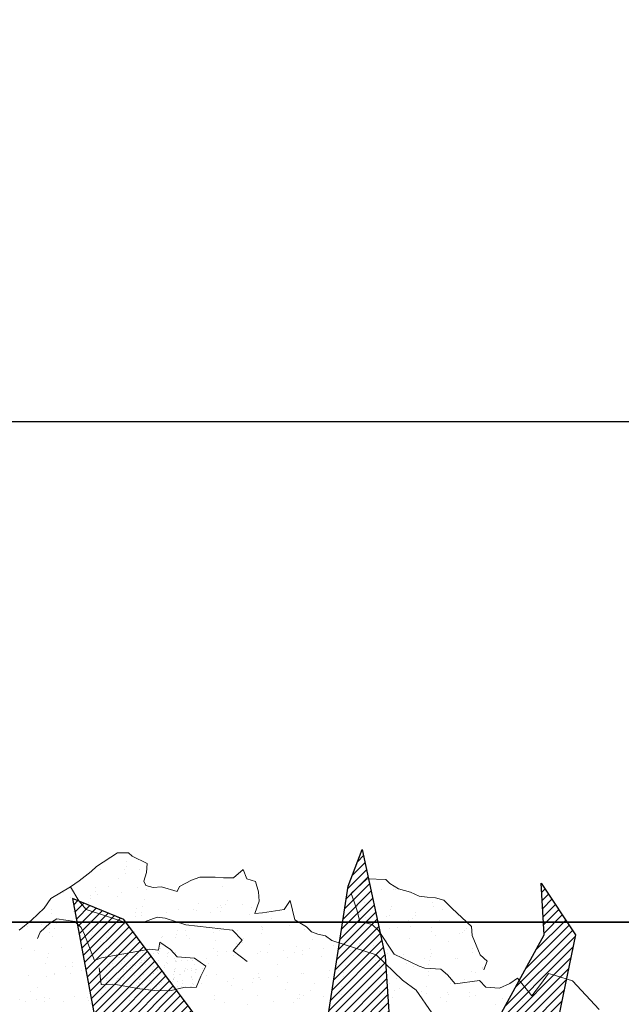
# Model space of a CAD drawing. Units: inches. Extents: x 1986 to 21484, y -1816 to 2016.
# Tile 77 of 85: x 3661 to 3676, y 1899 to 1924. Entities that reach past the tile are written whole.
import ezdxf

# ---------------------------------------------------------------- set-up
doc = ezdxf.new("R2010")
doc.units = ezdxf.units.IN
for name, color, linetype, lineweight in [('A-ANNO-DIMS', 2, 'Continuous', 18), ('C-PROP', 7, 'Continuous', 35), ('L-PLNT', 84, 'Continuous', 13), ('vfolhas', 114, 'Continuous', 5)]:
    doc.layers.add(name, color=color, linetype=linetype, lineweight=lineweight)
doc.layers.add('vfolha2', color=110, linetype='Continuous')
doc.layers.add('vfolhas2', color=102, linetype='Continuous')
doc.styles.get("Standard").update_dxf_attribs({"font": 'arial.ttf'})
doc.dimstyles.new('ISO-25', dxfattribs={"dimtxt": 8, "dimasz": 2.5, "dimexe": 1.25, "dimexo": 0.625, "dimtad": 1, "dimdec": 1, "dimlunit": 3, "dimtxsty": 'Standard', "dimcen": 2.5, "dimadec": 0, "dimazin": 0, "dimtfac": 1, "dimtdec": 1, "dimtmove": 0, "dimatfit": 3, "dimfxl": 1, "dimarcsym": 0})
pattern_1 = [(45, (-2446.5133113, 50.986076), (-0.004419417382, 0.004419417382), [])]

# ---------------------------------------------------------------- blocks, each defined once
blk = doc.blocks.new('*D33')
at = {"layer": 'A-ANNO-DIMS', "color": 0, "lineweight": -2, "transparency": 16777216}
for p, q in [((3538.907, 1901.377), (3538.907, 1914.655)), ((3898.907, 1901.377), (3898.907, 1914.655)), ((3541.407, 1913.405), (3896.407, 1913.405))]:
    blk.add_line(p, q, dxfattribs=at)
at = {"layer": 'A-ANNO-DIMS', "color": 0, "transparency": 16777216}
for points in [[(3541.407, 1913.821), (3541.407, 1912.988), (3538.907, 1913.405)], [(3896.407, 1913.821), (3896.407, 1912.988), (3898.907, 1913.405)]]:
    blk.add_solid(points, dxfattribs=at)
at = {"layer": 'Defpoints', "color": 0, "transparency": 16777216}
for p in [(3898.907, 1913.405), (3538.907, 1900.752), (3898.907, 1900.752)]:
    blk.add_point(p, dxfattribs=at)
at = {"layer": 'A-ANNO-DIMS', "color": 0, "transparency": 16777216, "insert": (3718.907, 1918.117), "char_height": 8, "attachment_point": 5}
blk.add_mtext("30'", dxfattribs=at)
blk = doc.blocks.new('arbusto_PB_verde_grande')
at = {"layer": 'vfolha2'}
h = blk.add_hatch(dxfattribs=at)
h.set_pattern_fill('ANSI31', color=256, scale=0.05, style=0)
h.set_pattern_definition(pattern_1)
h.paths.add_polyline_path([(0.0294, 0.3565), (0.0003, 0.0905), (0.0263, -0.0393), (0.047, 0.0623), (0.0619, 0.0973), (0.0937, 0.2657), (0.0996, 0.4347), (0.0879, 0.6131), (0.0645, 0.7227), (0.0499, 0.6851), (0.0236, 0.5129)])
h.paths.add_polyline_path([(0.3011, 0.4379), (0.1423, 0.2487), (0.2669, 0.3002)])
h.paths.add_polyline_path([(0.38, 0.2282), (0.237, 0.1519), (0.1843, 0.0936), (0.1112, 0.0436), (0.0263, -0.0393), (0.2806, 0.0467), (0.3683, 0.078), (0.4676, 0.1124), (0.6107, 0.1938), (0.7159, 0.2782), (0.5581, 0.2595)])
h.paths.add_polyline_path([(0.561, -0.2944), (0.7275, -0.3257), (0.5902, -0.2412), (0.4296, -0.1598), (0.0263, -0.0393), (0.1492, -0.1411), (0.1884, -0.166), (0.415, -0.2444)])
h.paths.add_polyline_path([(-0.2743, -0.4478), (-0.3035, -0.7263), (-0.2392, -0.6417), (-0.1546, -0.4572), (0.0263, -0.0393), (-0.1633, -0.2538)])
h.paths.add_polyline_path([(-0.5196, -0.2474), (-0.6774, -0.3257), (-0.5956, -0.3507), (-0.4057, -0.3288), (-0.2101, -0.21), (0.0263, -0.0393), (-0.1487, -0.0659), (-0.3152, -0.091), (-0.4145, -0.1505)])
h.paths.add_polyline_path([(-0.5255, 0.2501), (-0.7095, 0.247), (-0.5196, 0.1093), (-0.3298, 0.0217), (-0.0757, -0.0128), (-0.0423, -0.0215), (-0.3502, 0.1312)])
at = {"layer": 'vfolhas'}
h = blk.add_hatch(dxfattribs=at)
h.set_pattern_fill('ANSI31', color=256, scale=0.05, style=0)
h.set_pattern_definition(pattern_1)
h.paths.add_polyline_path([(-0.0728, 0.5067), (-0.1808, 0.6506), (-0.2334, 0.6725), (-0.2071, 0.5318), (-0.1078, 0.2501), (0.0263, -0.0393), (0.0003, 0.0905), (0.0082, 0.1624), (-0.0494, 0.2908)])
h.paths.add_polyline_path([(0.099, 0.4193), (0.0937, 0.2657), (0.0791, 0.1881), (0.1551, 0.369), (0.2661, 0.5505), (0.2836, 0.635), (0.2485, 0.6882), (0.2514, 0.635), (0.2018, 0.5443)])
h.paths.add_polyline_path([(0.1229, 0.2407), (0.047, 0.0623), (0.0263, -0.0393), (0.1112, 0.0436), (0.1843, 0.0936), (0.2748, 0.1938), (0.3215, 0.2532), (0.4413, 0.3847), (0.4763, 0.5787), (0.4179, 0.4535), (0.2894, 0.3095)])
h.paths.add_polyline_path([(0.5815, -0.0378), (0.7071, 0.0154), (0.7859, 0.0467), (0.748, 0.0655), (0.6282, 0.0842), (0.526, 0.0905), (0.3974, 0.0436), (0.0263, -0.0393), (0.2573, -0.0315), (0.4383, -0.0347)])
h.paths.add_polyline_path([(0.5202, -0.0365), (0.4383, -0.0347), (0.2573, -0.0315), (0.0263, -0.0393), (0.1796, -0.0852), (0.5377, -0.1317), (0.6954, -0.1536), (0.7859, -0.0785), (0.7041, -0.1004)])
h.paths.add_polyline_path([(0.2719, -0.2193), (0.1492, -0.1411), (0.0263, -0.0393), (0.1579, -0.3101), (0.2952, -0.4258), (0.4179, -0.4916), (0.564, -0.5667), (0.5114, -0.4853), (0.3946, -0.3414)])
h.paths.add_polyline_path([(-0.0582, -0.4759), (-0.0231, -0.6198), (0.047, -0.8013), (0.0849, -0.5979), (0.0791, -0.4071), (0.0353, -0.2538), (0.0263, -0.0393), (-0.0377, -0.26)])
h.paths.add_polyline_path([(-0.2422, 0.1405), (-0.1107, 0.0686), (0.0263, -0.0393), (-0.0423, 0.1087), (-0.2101, 0.2376), (-0.3649, 0.3314), (-0.4787, 0.4034), (-0.543, 0.4629), (-0.4904, 0.3314), (-0.3941, 0.2219)])
at = {"layer": 'vfolha2'}
for p, q in [((0.0499, 0.6851), (0.0645, 0.7227)), ((0.0645, 0.7227), (0.0879, 0.6131)), ((0.0236, 0.5129), (0.0499, 0.6851)), ((0.0879, 0.6131), (0.0996, 0.4347))]:
    blk.add_line(p, q, dxfattribs=at)
at = {"layer": 'vfolhas2'}
for p, q in [((0.2514, 0.635), (0.2485, 0.6882)), ((0.2485, 0.6882), (0.2836, 0.635)), ((-0.2334, 0.6725), (-0.2071, 0.5318)), ((-0.1808, 0.6506), (-0.2334, 0.6725)), ((-0.0728, 0.5067), (-0.1808, 0.6506)), ((0.2018, 0.5443), (0.2514, 0.635)), ((0.2836, 0.635), (0.2661, 0.5505))]:
    blk.add_line(p, q, dxfattribs=at)
blk = doc.blocks.new('PLANT-SHRUB')
for p, q in [((2149.028, 1883.988), (2149.028, 1883.002)), ((2149.028, 1883.002), (2149.248, 1882.608)), ((2149.248, 1882.608), (2149.341, 1882.445)), ((2149.341, 1882.445), (2149.678, 1882.515)), ((2149.341, 1882.445), (2149.341, 1882.445)), ((2149.678, 1882.515), (2150.037, 1882.573)), ((2150.037, 1882.573), (2149.992, 1881.999)), ((2150.304, 1882.515), (2150.304, 1882.515)), ((2149.992, 1881.999), (2150.224, 1881.964)), ((2150.224, 1881.964), (2150.503, 1881.872)), ((2150.62, 1882.101), (2150.62, 1882.101)), ((2150.843, 1882.101), (2150.843, 1882.101)), ((2150.503, 1881.872), (2150.735, 1881.616)), ((2150.735, 1881.616), (2150.735, 1881.384)), ((2151.073, 1881.595), (2151.073, 1881.595)), ((2151.203, 1881.501), (2151.203, 1881.501)), ((2150.26, 1881.16), (2150.471, 1881.261)), ((2150.466, 1881.208), (2150.466, 1881.208)), ((2150.735, 1881.384), (2151.241, 1881.026)), ((2150.818, 1881.331), (2150.818, 1881.331)), ((2151.13, 1881.433), (2151.13, 1881.433)), ((2151.71, 1881.206), (2151.71, 1881.206)), ((2150.26, 1881.16), (2150.26, 1881.16)), ((2150.279, 1880.922), (2150.26, 1881.16)), ((2150.458, 1881.185), (2150.458, 1881.185)), ((2150.666, 1881.157), (2150.666, 1881.157)), ((2150.732, 1881.068), (2150.732, 1881.068)), ((2150.991, 1881.114), (2150.991, 1881.114)), ((2151.241, 1881.026), (2151.223, 1880.723)), ((2151.534, 1881.043), (2151.534, 1881.043)), ((2151.542, 1881.098), (2151.542, 1881.098)), ((2151.742, 1881.016), (2151.742, 1881.016)), ((2152.069, 1880.464), (2152.174, 1881.154)), ((2150.086, 1880.427), (2150.279, 1880.922)), ((2150.384, 1880.75), (2150.384, 1880.75)), ((2151.223, 1880.723), (2151.251, 1880.503)), ((2151.333, 1880.936), (2151.333, 1880.936)), ((2151.933, 1880.718), (2151.933, 1880.718)), ((2150.31, 1880.682), (2150.31, 1880.682)), ((2150.75, 1880.594), (2150.75, 1880.594)), ((2150.793, 1880.561), (2150.793, 1880.561)), ((2151.251, 1880.503), (2151.526, 1880.21)), ((2151.815, 1880.566), (2151.815, 1880.566)), ((2151.994, 1880.591), (2151.994, 1880.591)), ((2152.153, 1880.045), (2152.069, 1880.464)), ((2149.949, 1880.253), (2150.086, 1880.427)), ((2149.949, 1880.253), (2149.949, 1880.253)), ((2149.994, 1879.584), (2149.949, 1880.253)), ((2150.143, 1880.207), (2150.143, 1880.207)), ((2150.228, 1880.204), (2150.228, 1880.204)), ((2151.388, 1880.205), (2151.388, 1880.205)), ((2151.512, 1880.332), (2151.512, 1880.332)), ((2151.526, 1880.21), (2151.599, 1880.073)), ((2151.586, 1880.399), (2151.586, 1880.399)), ((2152.632, 1880.203), (2152.632, 1880.203)), ((2150.089, 1880.198), (2150.089, 1880.198)), ((2150.297, 1880.171), (2150.297, 1880.171)), ((2150.622, 1880.128), (2150.622, 1880.128)), ((2151.114, 1879.967), (2151.114, 1879.967)), ((2151.165, 1880.057), (2151.165, 1880.057)), ((2151.219, 1880.098), (2151.219, 1880.098)), ((2151.308, 1880.165), (2151.308, 1880.165)), ((2151.373, 1880.029), (2151.373, 1880.029)), ((2151.599, 1880.073), (2151.856, 1879.419)), ((2151.698, 1879.986), (2151.698, 1879.986)), ((2152.153, 1880.045), (2152.153, 1880.045)), ((2152.195, 1879.125), (2152.153, 1880.045)), ((2152.354, 1880.152), (2152.354, 1880.152)), ((2152.464, 1880.095), (2152.464, 1880.095)), ((2152.713, 1879.981), (2152.713, 1879.981)), ((2152.787, 1880.048), (2152.787, 1880.048)), ((2150.767, 1879.791), (2150.767, 1879.791)), ((2151.79, 1879.796), (2151.79, 1879.796)), ((2152.241, 1879.915), (2152.241, 1879.915)), ((2152.449, 1879.888), (2152.449, 1879.888)), ((2152.774, 1879.845), (2152.774, 1879.845)), ((2152.869, 1879.757), (2152.869, 1879.757)), ((2153.317, 1879.773), (2153.317, 1879.773)), ((2150.004, 1879.282), (2149.994, 1879.584)), ((2150.427, 1879.593), (2150.427, 1879.593)), ((2150.693, 1879.581), (2150.693, 1879.581)), ((2150.766, 1879.648), (2150.766, 1879.648)), ((2151.672, 1879.591), (2151.672, 1879.591)), ((2152.316, 1879.616), (2152.316, 1879.616)), ((2152.916, 1879.588), (2152.916, 1879.588)), ((2150.114, 1879.098), (2150.004, 1879.282)), ((2150.203, 1879.434), (2150.203, 1879.434)), ((2150.295, 1879.216), (2150.295, 1879.216)), ((2151.065, 1879.204), (2151.065, 1879.204)), ((2151.283, 1879.395), (2151.283, 1879.395)), ((2151.856, 1879.419), (2151.728, 1878.713)), ((2151.894, 1879.23), (2151.894, 1879.23)), ((2151.968, 1879.298), (2151.968, 1879.298)), ((2152.329, 1879.382), (2152.329, 1879.382)), ((2153.351, 1879.387), (2153.351, 1879.387)), ((2153.517, 1879.266), (2153.517, 1879.266)), ((2150.26, 1878.943), (2150.114, 1879.098)), ((2150.254, 1879.142), (2150.254, 1879.142)), ((2150.742, 1879.021), (2150.742, 1879.021)), ((2150.797, 1879.07), (2150.797, 1879.07)), ((2150.896, 1879.097), (2150.896, 1879.097)), ((2151.005, 1879.043), (2151.005, 1879.043)), ((2151.33, 1879), (2151.33, 1879)), ((2151.765, 1879.026), (2151.765, 1879.026)), ((2152.141, 1879.094), (2152.141, 1879.094)), ((2152.195, 1879.125), (2152.195, 1879.125)), ((2152.763, 1878.087), (2152.195, 1879.125)), ((2152.31, 1879.202), (2152.31, 1879.202)), ((2152.844, 1878.987), (2152.844, 1878.987)), ((2153.386, 1879.092), (2153.386, 1879.092)), ((2153.554, 1879.2), (2153.554, 1879.2)), ((2153.89, 1878.973), (2153.89, 1878.973)), ((2150.389, 1878.787), (2150.26, 1878.943)), ((2150.48, 1878.558), (2150.389, 1878.787)), ((2151.496, 1878.866), (2151.496, 1878.866)), ((2151.728, 1878.713), (2151.746, 1878.494)), ((2151.873, 1878.929), (2151.873, 1878.929)), ((2152.081, 1878.901), (2152.081, 1878.901)), ((2152.406, 1878.859), (2152.406, 1878.859)), ((2152.948, 1878.787), (2152.948, 1878.787)), ((2153.096, 1878.879), (2153.096, 1878.879)), ((2153.156, 1878.76), (2153.156, 1878.76)), ((2153.169, 1878.947), (2153.169, 1878.947)), ((2153.481, 1878.717), (2153.481, 1878.717)), ((2150.646, 1878.292), (2150.48, 1878.558)), ((2151.075, 1878.48), (2151.075, 1878.48)), ((2151.149, 1878.547), (2151.149, 1878.547)), ((2151.258, 1878.625), (2151.258, 1878.625)), ((2151.349, 1878.59), (2151.349, 1878.59)), ((2151.746, 1878.494), (2151.92, 1878.228)), ((2152.304, 1878.612), (2152.304, 1878.612)), ((2152.594, 1878.588), (2152.594, 1878.588)), ((2152.698, 1878.515), (2152.698, 1878.515)), ((2153.326, 1878.617), (2153.326, 1878.617)), ((2153.838, 1878.585), (2153.838, 1878.585)), ((2154.024, 1878.645), (2154.024, 1878.645)), ((2154.232, 1878.618), (2154.232, 1878.618)), ((2154.297, 1878.529), (2154.297, 1878.529)), ((2154.371, 1878.596), (2154.371, 1878.596)), ((2154.406, 1878.578), (2154.406, 1878.578)), ((2154.557, 1878.575), (2154.557, 1878.575)), ((2150.71, 1878.044), (2150.646, 1878.292)), ((2150.717, 1878.251), (2150.717, 1878.251)), ((2151.739, 1878.255), (2151.739, 1878.255)), ((2151.92, 1878.228), (2151.774, 1877.953)), ((2152.819, 1878.217), (2152.819, 1878.217)), ((2154.888, 1878.208), (2154.888, 1878.208)), ((2150.71, 1877.898), (2150.71, 1878.044)), ((2150.742, 1878.203), (2150.742, 1878.203)), ((2150.961, 1878.014), (2150.961, 1878.014)), ((2151.818, 1878.094), (2151.818, 1878.094)), ((2152.8, 1877.891), (2152.763, 1878.087)), ((2153.063, 1878.091), (2153.063, 1878.091)), ((2153.231, 1878.199), (2153.231, 1878.199)), ((2153.865, 1878.203), (2153.865, 1878.203)), ((2153.899, 1878.164), (2153.899, 1878.164)), ((2154.307, 1878.089), (2154.307, 1878.089)), ((2154.476, 1878.196), (2154.476, 1878.196)), ((2151.058, 1877.559), (2150.71, 1877.898)), ((2151.232, 1877.855), (2151.232, 1877.855)), ((2151.504, 1877.942), (2151.504, 1877.942)), ((2151.682, 1877.76), (2151.599, 1877.559)), ((2151.774, 1877.953), (2151.682, 1877.76)), ((2151.712, 1877.915), (2151.712, 1877.915)), ((2152.916, 1877.731), (2152.8, 1877.891)), ((2152.996, 1877.578), (2152.916, 1877.731)), ((2153.113, 1877.731), (2153.113, 1877.731)), ((2153.301, 1877.847), (2153.301, 1877.847)), ((2153.478, 1877.778), (2153.478, 1877.778)), ((2153.552, 1877.845), (2153.552, 1877.845)), ((2154.38, 1877.808), (2154.38, 1877.808)), ((2155.101, 1877.813), (2155.101, 1877.813)), ((2155.427, 1877.795), (2155.427, 1877.795)), ((2151.058, 1877.559), (2151.058, 1877.559)), ((2151.599, 1877.559), (2151.058, 1877.559)), ((2152.996, 1877.396), (2152.996, 1877.578)), ((2153.515, 1877.584), (2153.515, 1877.584)), ((2153.656, 1877.659), (2153.656, 1877.659)), ((2153.864, 1877.632), (2153.864, 1877.632)), ((2154.189, 1877.589), (2154.189, 1877.589)), ((2154.732, 1877.518), (2154.732, 1877.518)), ((2154.753, 1877.495), (2154.753, 1877.495)), ((2154.76, 1877.582), (2154.76, 1877.582)), ((2154.94, 1877.49), (2154.94, 1877.49)), ((2153.091, 1877.069), (2152.996, 1877.396)), ((2153.08, 1877.413), (2153.08, 1877.413)), ((2153.84, 1877.433), (2153.84, 1877.433)), ((2154.679, 1877.427), (2154.679, 1877.427)), ((2154.862, 1877.438), (2154.862, 1877.438)), ((2155.265, 1877.447), (2155.265, 1877.447)), ((2155.807, 1877.376), (2155.807, 1877.376)), ((2152.844, 1876.63), (2153.091, 1877.069)), ((2153.276, 1877.077), (2153.276, 1877.077)), ((2153.985, 1877.088), (2153.985, 1877.088)), ((2154.153, 1877.196), (2154.153, 1877.196)), ((2154.282, 1877.063), (2154.282, 1877.063)), ((2154.355, 1877.038), (2154.355, 1877.038)), ((2154.764, 1876.572), (2154.691, 1877.009)), ((2155.229, 1877.086), (2155.229, 1877.086)), ((2155.398, 1877.193), (2155.398, 1877.193)), ((2155.401, 1877.024), (2155.401, 1877.024)), ((2155.881, 1877.076), (2155.881, 1877.076)), ((2155.955, 1877.144), (2155.955, 1877.144)), ((2153.934, 1876.744), (2153.934, 1876.744)), ((2153.107, 1876.695), (2152.844, 1876.63)), ((2153.565, 1876.375), (2153.107, 1876.695)), ((2153.495, 1876.645), (2153.495, 1876.645)), ((2153.815, 1876.663), (2153.815, 1876.663)), ((2153.82, 1876.603), (2153.82, 1876.603)), ((2153.86, 1876.677), (2153.86, 1876.677)), ((2154.363, 1876.531), (2154.363, 1876.531)), ((2154.414, 1876.528), (2154.764, 1876.572)), ((2154.414, 1876.179), (2154.414, 1876.528)), ((2154.437, 1876.581), (2154.437, 1876.581)), ((2154.571, 1876.504), (2154.571, 1876.504)), ((2154.837, 1876.668), (2154.837, 1876.668)), ((2155.483, 1876.712), (2155.483, 1876.712)), ((2155.535, 1876.382), (2155.8, 1876.479)), ((2155.682, 1876.579), (2155.682, 1876.579)), ((2155.8, 1876.479), (2156.079, 1876.605)), ((2155.917, 1876.629), (2155.917, 1876.629)), ((2156.068, 1876.514), (2156.068, 1876.514)), ((2156.074, 1876.482), (2156.074, 1876.482)), ((2156.079, 1876.605), (2156.274, 1876.41)), ((2156.151, 1876.503), (2156.151, 1876.503)), ((2156.165, 1876.486), (2156.165, 1876.486)), ((2153.42, 1876.106), (2153.718, 1876.259)), ((2153.565, 1876.375), (2153.565, 1876.375)), ((2153.718, 1876.259), (2153.565, 1876.375)), ((2154.33, 1876.268), (2154.33, 1876.268)), ((2154.896, 1876.461), (2154.896, 1876.461)), ((2155.062, 1876.326), (2155.062, 1876.326)), ((2155.135, 1876.393), (2155.135, 1876.393)), ((2155.376, 1876.254), (2155.376, 1876.254)), ((2155.439, 1876.39), (2155.439, 1876.39)), ((2155.605, 1876.034), (2155.535, 1876.382)), ((2155.594, 1876.403), (2155.594, 1876.403)), ((2155.647, 1876.362), (2155.647, 1876.362)), ((2155.764, 1876.284), (2155.764, 1876.284)), ((2155.787, 1876.255), (2155.787, 1876.255)), ((2155.831, 1876.327), (2155.831, 1876.327)), ((2155.972, 1876.319), (2155.972, 1876.319)), ((2156.006, 1876.34), (2156.006, 1876.34)), ((2156.013, 1876.397), (2156.013, 1876.397)), ((2156.219, 1876.239), (2156.219, 1876.239)), ((2156.262, 1876.284), (2156.262, 1876.284)), ((2156.274, 1876.41), (2156.622, 1876.215)), ((2156.329, 1876.327), (2156.329, 1876.327)), ((2156.399, 1876.259), (2156.399, 1876.259)), ((2156.515, 1876.248), (2156.515, 1876.248)), ((2156.685, 1876.361), (2156.685, 1876.361)), ((2156.723, 1876.221), (2156.723, 1876.221)), ((2153.274, 1875.924), (2153.42, 1876.106)), ((2153.662, 1876.087), (2153.662, 1876.087)), ((2153.83, 1876.195), (2153.83, 1876.195)), ((2155.187, 1875.275), (2154.414, 1876.179)), ((2154.907, 1876.085), (2154.907, 1876.085)), ((2155.075, 1876.193), (2155.075, 1876.193)), ((2155.605, 1876.034), (2155.605, 1876.034)), ((2155.898, 1875.713), (2155.605, 1876.034)), ((2155.678, 1876.04), (2155.678, 1876.04)), ((2155.703, 1876.148), (2155.703, 1876.148)), ((2155.837, 1876.185), (2155.837, 1876.185)), ((2155.867, 1876.212), (2155.867, 1876.212)), ((2155.92, 1876.119), (2155.92, 1876.119)), ((2155.945, 1876.082), (2155.945, 1876.082)), ((2156.003, 1876.089), (2156.003, 1876.089)), ((2156.004, 1876.108), (2156.004, 1876.108)), ((2156.134, 1876.091), (2156.134, 1876.091)), ((2156.151, 1876.083), (2156.151, 1876.083)), ((2156.263, 1875.975), (2156.263, 1875.975)), ((2156.318, 1876.045), (2156.318, 1876.045)), ((2156.32, 1876.19), (2156.32, 1876.19)), ((2156.337, 1876.042), (2156.337, 1876.042)), ((2156.347, 1876.072), (2156.347, 1876.072)), ((2156.351, 1876.063), (2156.351, 1876.063)), ((2156.412, 1876.091), (2156.412, 1876.091)), ((2156.434, 1876.052), (2156.434, 1876.052)), ((2156.443, 1876.081), (2156.443, 1876.081)), ((2156.486, 1876.2), (2156.486, 1876.2)), ((2156.564, 1876.035), (2156.564, 1876.035)), ((2156.622, 1876.215), (2156.901, 1875.936)), ((2156.622, 1876.215), (2156.622, 1876.215)), ((2156.781, 1876.006), (2156.781, 1876.006)), ((2157.048, 1876.178), (2157.048, 1876.178)), ((2153.15, 1875.678), (2153.274, 1875.924)), ((2153.79, 1875.893), (2153.79, 1875.893)), ((2154.664, 1875.961), (2154.664, 1875.961)), ((2154.812, 1875.898), (2154.812, 1875.898)), ((2155.702, 1875.927), (2155.702, 1875.927)), ((2155.777, 1875.947), (2155.777, 1875.947)), ((2155.891, 1875.859), (2155.891, 1875.859)), ((2155.99, 1875.745), (2155.99, 1875.745)), ((2155.993, 1875.781), (2155.993, 1875.781)), ((2156.02, 1875.772), (2156.02, 1875.772)), ((2156.133, 1875.883), (2156.133, 1875.883)), ((2156.159, 1875.899), (2156.159, 1875.899)), ((2156.2, 1875.926), (2156.2, 1875.926)), ((2156.209, 1875.931), (2156.209, 1875.931)), ((2156.402, 1875.783), (2156.402, 1875.783)), ((2156.627, 1875.926), (2156.627, 1875.926)), ((2156.631, 1875.882), (2156.631, 1875.882)), ((2156.639, 1875.759), (2156.639, 1875.759)), ((2156.698, 1875.925), (2156.698, 1875.925)), ((2156.798, 1875.905), (2156.798, 1875.905)), ((2156.828, 1875.932), (2156.828, 1875.932)), ((2156.833, 1875.768), (2156.833, 1875.768)), ((2156.901, 1875.936), (2157.138, 1875.658)), ((2156.938, 1875.846), (2156.938, 1875.846)), ((2153.15, 1875.678), (2153.15, 1875.678)), ((2153.264, 1875.481), (2153.15, 1875.678)), ((2153.171, 1875.243), (2153.264, 1875.481)), ((2153.264, 1875.481), (2153.264, 1875.481)), ((2153.995, 1875.545), (2153.995, 1875.545)), ((2154.114, 1875.581), (2154.114, 1875.581)), ((2154.203, 1875.518), (2154.203, 1875.518)), ((2154.243, 1875.575), (2154.243, 1875.575)), ((2154.305, 1875.498), (2154.305, 1875.498)), ((2154.316, 1875.643), (2154.316, 1875.643)), ((2154.528, 1875.475), (2154.528, 1875.475)), ((2155.351, 1875.484), (2155.351, 1875.484)), ((2155.359, 1875.578), (2155.359, 1875.578)), ((2155.865, 1875.61), (2155.865, 1875.61)), ((2155.898, 1875.463), (2155.898, 1875.713)), ((2155.983, 1875.473), (2155.983, 1875.473)), ((2155.986, 1875.697), (2155.986, 1875.697)), ((2156.004, 1875.483), (2156.004, 1875.483)), ((2156.071, 1875.526), (2156.071, 1875.526)), ((2156.199, 1875.623), (2156.199, 1875.623)), ((2156.203, 1875.668), (2156.203, 1875.668)), ((2156.286, 1875.657), (2156.286, 1875.657)), ((2156.314, 1875.68), (2156.314, 1875.68)), ((2156.373, 1875.489), (2156.373, 1875.489)), ((2156.392, 1875.475), (2156.392, 1875.475)), ((2156.416, 1875.64), (2156.416, 1875.64)), ((2156.471, 1875.605), (2156.471, 1875.605)), ((2156.5, 1875.632), (2156.5, 1875.632)), ((2156.501, 1875.482), (2156.501, 1875.482)), ((2156.569, 1875.525), (2156.569, 1875.525)), ((2156.604, 1875.576), (2156.604, 1875.576)), ((2156.617, 1875.618), (2156.617, 1875.618)), ((2156.634, 1875.611), (2156.634, 1875.611)), ((2156.717, 1875.6), (2156.717, 1875.6)), ((2156.812, 1875.68), (2156.812, 1875.68)), ((2156.847, 1875.583), (2156.847, 1875.583)), ((2156.981, 1875.491), (2156.981, 1875.491)), ((2156.999, 1875.481), (2156.999, 1875.481)), ((2157.026, 1875.62), (2157.026, 1875.62)), ((2157.064, 1875.555), (2157.064, 1875.555)), ((2157.067, 1875.524), (2157.067, 1875.524)), ((2157.12, 1875.619), (2157.12, 1875.619)), ((2157.138, 1875.658), (2157.486, 1875.198)), ((2157.147, 1875.544), (2157.147, 1875.544)), ((2157.465, 1875.624), (2157.465, 1875.624)), ((2157.538, 1875.692), (2157.538, 1875.692)), ((2153.492, 1875.233), (2153.171, 1875.243)), ((2153.678, 1875.057), (2153.492, 1875.233)), ((2155.07, 1875.403), (2155.07, 1875.403)), ((2155.449, 1874.794), (2155.187, 1875.275)), ((2155.278, 1875.376), (2155.278, 1875.376)), ((2155.444, 1875.224), (2155.444, 1875.224)), ((2155.518, 1875.292), (2155.518, 1875.292)), ((2155.603, 1875.333), (2155.603, 1875.333)), ((2155.967, 1875.142), (2155.898, 1875.463)), ((2156.134, 1875.268), (2155.967, 1875.142)), ((2156.056, 1875.274), (2156.056, 1875.274)), ((2156.274, 1875.101), (2156.134, 1875.268)), ((2156.139, 1875.263), (2156.139, 1875.263)), ((2156.143, 1875.304), (2156.143, 1875.304)), ((2156.146, 1875.262), (2156.146, 1875.262)), ((2156.173, 1875.331), (2156.173, 1875.331)), ((2156.185, 1875.28), (2156.185, 1875.28)), ((2156.189, 1875.315), (2156.189, 1875.315)), ((2156.269, 1875.245), (2156.269, 1875.245)), ((2156.312, 1875.459), (2156.312, 1875.459)), ((2156.354, 1875.234), (2156.354, 1875.234)), ((2156.607, 1875.31), (2156.607, 1875.31)), ((2156.682, 1875.279), (2156.682, 1875.279)), ((2156.792, 1875.318), (2156.792, 1875.318)), ((2156.823, 1875.46), (2156.823, 1875.46)), ((2156.951, 1875.464), (2156.951, 1875.464)), ((2157.016, 1875.312), (2157.016, 1875.312)), ((2157.067, 1875.26), (2157.067, 1875.26)), ((2157.18, 1875.278), (2157.18, 1875.278)), ((2157.242, 1875.454), (2157.242, 1875.454)), ((2157.453, 1875.45), (2157.453, 1875.45)), ((2153.823, 1874.902), (2153.678, 1875.057)), ((2153.845, 1875.211), (2153.845, 1875.211)), ((2154.584, 1875.084), (2154.584, 1875.084)), ((2154.752, 1875.192), (2154.752, 1875.192)), ((2154.787, 1875.128), (2154.787, 1875.128)), ((2155.828, 1875.082), (2155.828, 1875.082)), ((2155.866, 1875.089), (2155.866, 1875.089)), ((2155.967, 1875.142), (2155.967, 1875.142)), ((2155.972, 1875.165), (2155.972, 1875.165)), ((2155.984, 1875.159), (2155.984, 1875.159)), ((2155.997, 1875.19), (2155.997, 1875.19)), ((2156.873, 1874.711), (2156.274, 1875.101)), ((2156.372, 1875.082), (2156.372, 1875.082)), ((2156.381, 1875.167), (2156.381, 1875.167)), ((2156.44, 1875.125), (2156.44, 1875.125)), ((2156.465, 1875.018), (2156.465, 1875.018)), ((2156.486, 1875.217), (2156.486, 1875.217)), ((2156.569, 1875.206), (2156.569, 1875.206)), ((2156.597, 1875.002), (2156.597, 1875.002)), ((2156.624, 1875.164), (2156.624, 1875.164)), ((2156.653, 1875.191), (2156.653, 1875.191)), ((2156.679, 1875.191), (2156.679, 1875.191)), ((2156.699, 1875.189), (2156.699, 1875.189)), ((2156.813, 1875.152), (2156.813, 1875.152)), ((2156.87, 1875.081), (2156.87, 1875.081)), ((2156.912, 1875.076), (2156.912, 1875.076)), ((2156.917, 1875.16), (2156.917, 1875.16)), ((2156.938, 1875.124), (2156.938, 1875.124)), ((2157, 1875.149), (2157, 1875.149)), ((2157.006, 1875.004), (2157.006, 1875.004)), ((2157.073, 1875.08), (2157.073, 1875.08)), ((2157.104, 1875.024), (2157.104, 1875.024)), ((2157.13, 1875.132), (2157.13, 1875.132)), ((2157.134, 1875.051), (2157.134, 1875.051)), ((2157.222, 1875.12), (2157.222, 1875.12)), ((2157.232, 1875.146), (2157.232, 1875.146)), ((2157.242, 1875.187), (2157.242, 1875.187)), ((2157.273, 1875.178), (2157.273, 1875.178)), ((2157.347, 1875.104), (2157.347, 1875.104)), ((2157.368, 1875.08), (2157.368, 1875.08)), ((2157.43, 1875.093), (2157.43, 1875.093)), ((2157.43, 1875.093), (2157.43, 1875.093)), ((2157.435, 1875.123), (2157.435, 1875.123)), ((2157.438, 1874.988), (2157.438, 1874.988)), ((2157.486, 1875.198), (2157.779, 1874.906)), ((2157.56, 1875.076), (2157.56, 1875.076)), ((2157.755, 1875.05), (2157.755, 1875.05)), ((2157.935, 1875.08), (2157.935, 1875.08)), ((2158.298, 1874.978), (2158.298, 1874.978)), ((2158.318, 1875.078), (2158.318, 1875.078)), ((2154.103, 1874.633), (2153.823, 1874.902)), ((2155.046, 1874.86), (2155.046, 1874.86)), ((2155.58, 1874.634), (2155.449, 1874.794)), ((2156.645, 1874.874), (2156.645, 1874.874)), ((2156.719, 1874.941), (2156.719, 1874.941)), ((2156.803, 1874.844), (2156.803, 1874.844)), ((2156.852, 1874.755), (2156.852, 1874.755)), ((2156.945, 1874.878), (2156.945, 1874.878)), ((2156.982, 1874.738), (2156.982, 1874.738)), ((2157.051, 1874.878), (2157.051, 1874.878)), ((2157.222, 1874.838), (2157.222, 1874.838)), ((2157.426, 1874.738), (2157.426, 1874.738)), ((2157.779, 1874.906), (2157.528, 1874.571)), ((2157.549, 1874.877), (2157.549, 1874.877)), ((2157.585, 1874.883), (2157.585, 1874.883)), ((2157.614, 1874.91), (2157.614, 1874.91)), ((2157.631, 1874.84), (2157.631, 1874.84)), ((2158.268, 1874.909), (2158.268, 1874.909)), ((2154.31, 1874.55), (2154.103, 1874.633)), ((2154.641, 1874.457), (2154.31, 1874.55)), ((2154.766, 1874.509), (2154.641, 1874.457)), ((2154.974, 1874.153), (2154.766, 1874.509)), ((2155.326, 1874.714), (2155.326, 1874.714)), ((2155.901, 1874.503), (2155.58, 1874.634)), ((2156.28, 1874.139), (2155.901, 1874.503)), ((2156.248, 1874.509), (2156.248, 1874.509)), ((2156.281, 1874.575), (2156.281, 1874.575)), ((2156.348, 1874.719), (2156.348, 1874.719)), ((2157.309, 1874.42), (2156.873, 1874.711)), ((2156.996, 1874.696), (2156.996, 1874.696)), ((2157.199, 1874.709), (2157.199, 1874.709)), ((2157.239, 1874.68), (2157.239, 1874.68)), ((2157.283, 1874.698), (2157.283, 1874.698)), ((2157.287, 1874.61), (2157.287, 1874.61)), ((2157.306, 1874.723), (2157.306, 1874.723)), ((2157.413, 1874.681), (2157.413, 1874.681)), ((2157.428, 1874.68), (2157.428, 1874.68)), ((2157.428, 1874.68), (2157.428, 1874.68)), ((2157.526, 1874.573), (2157.526, 1874.573)), ((2157.528, 1874.571), (2157.585, 1874.647)), ((2157.847, 1874.523), (2157.847, 1874.523)), ((2157.921, 1874.59), (2157.921, 1874.59)), ((2158.474, 1874.667), (2158.474, 1874.667)), ((2158.77, 1874.571), (2158.77, 1874.571)), ((2155.778, 1874.275), (2155.778, 1874.275)), ((2155.841, 1874.319), (2155.841, 1874.319)), ((2155.986, 1874.248), (2155.986, 1874.248)), ((2156.887, 1874.305), (2156.887, 1874.305)), ((2157.221, 1873.694), (2157.486, 1874.349)), ((2157.309, 1874.42), (2157.309, 1874.42)), ((2157.486, 1874.349), (2157.309, 1874.42)), ((2157.91, 1874.31), (2157.91, 1874.31)), ((2158.989, 1874.271), (2158.989, 1874.271)), ((2159.122, 1874.24), (2159.122, 1874.24)), ((2155.14, 1874.018), (2154.974, 1874.153)), ((2155.244, 1873.853), (2155.14, 1874.018)), ((2155.506, 1874.081), (2155.506, 1874.081)), ((2155.674, 1874.189), (2155.674, 1874.189)), ((2155.826, 1874.123), (2155.826, 1874.123)), ((2155.9, 1874.19), (2155.9, 1874.19)), ((2156.514, 1873.716), (2156.28, 1874.139)), ((2156.311, 1874.205), (2156.311, 1874.205)), ((2156.75, 1874.079), (2156.75, 1874.079)), ((2156.854, 1874.134), (2156.854, 1874.134)), ((2156.919, 1874.186), (2156.919, 1874.186)), ((2157.062, 1874.106), (2157.062, 1874.106)), ((2157.387, 1874.064), (2157.387, 1874.064)), ((2157.449, 1874.158), (2157.449, 1874.158)), ((2157.929, 1873.992), (2157.929, 1873.992)), ((2157.995, 1874.077), (2157.995, 1874.077)), ((2158.163, 1874.184), (2158.163, 1874.184)), ((2159.048, 1874.172), (2159.048, 1874.172)), ((2159.24, 1874.075), (2159.24, 1874.075)), ((2155.005, 1873.625), (2155.202, 1873.739)), ((2155.202, 1873.739), (2155.244, 1873.853)), ((2155.301, 1873.944), (2155.301, 1873.944)), ((2155.428, 1873.758), (2155.428, 1873.758)), ((2156.323, 1873.949), (2156.323, 1873.949)), ((2157.028, 1873.772), (2157.028, 1873.772)), ((2157.101, 1873.84), (2157.101, 1873.84)), ((2157.403, 1873.91), (2157.403, 1873.91)), ((2158.137, 1873.965), (2158.137, 1873.965)), ((2158.449, 1873.897), (2158.449, 1873.897)), ((2158.462, 1873.922), (2158.462, 1873.922)), ((2158.651, 1873.807), (2158.651, 1873.807)), ((2159.005, 1873.85), (2159.005, 1873.85)), ((2159.213, 1873.823), (2159.213, 1873.823)), ((2159.471, 1873.902), (2159.471, 1873.902)), ((2159.538, 1873.78), (2159.538, 1873.78)), ((2154.84, 1873.47), (2155.005, 1873.625)), ((2155.005, 1873.625), (2155.005, 1873.625)), ((2155.816, 1873.549), (2155.816, 1873.549)), ((2155.958, 1873.574), (2155.958, 1873.574)), ((2156.762, 1873.265), (2156.514, 1873.716)), ((2156.862, 1873.535), (2156.862, 1873.535)), ((2157.166, 1873.513), (2157.221, 1873.694)), ((2157.18, 1873.29), (2157.166, 1873.513)), ((2157.203, 1873.572), (2157.203, 1873.572)), ((2157.885, 1873.54), (2157.885, 1873.54)), ((2158.303, 1873.489), (2158.303, 1873.489)), ((2158.447, 1873.57), (2158.447, 1873.57)), ((2158.964, 1873.501), (2158.964, 1873.501)), ((2154.985, 1873.077), (2154.84, 1873.47)), ((2155.081, 1873.44), (2155.081, 1873.44)), ((2155.409, 1873.289), (2155.409, 1873.289)), ((2155.617, 1873.262), (2155.617, 1873.262)), ((2156.63, 1873.408), (2156.63, 1873.408)), ((2156.746, 1872.977), (2156.762, 1873.265)), ((2157.458, 1872.928), (2157.18, 1873.29)), ((2158.229, 1873.421), (2158.229, 1873.421)), ((2154.995, 1872.952), (2154.985, 1873.077)), ((2155.183, 1873.081), (2155.183, 1873.081)), ((2155.276, 1873.174), (2155.276, 1873.174)), ((2155.351, 1873.188), (2155.351, 1873.188)), ((2155.942, 1873.219), (2155.942, 1873.219)), ((2156.209, 1873.022), (2156.209, 1873.022)), ((2156.282, 1873.089), (2156.282, 1873.089)), ((2156.298, 1873.179), (2156.298, 1873.179)), ((2156.427, 1873.078), (2156.427, 1873.078)), ((2156.485, 1873.147), (2156.485, 1873.147)), ((2156.596, 1873.186), (2156.596, 1873.186)), ((2156.693, 1873.12), (2156.693, 1873.12)), ((2157.018, 1873.077), (2157.018, 1873.077)), ((2157.377, 1873.14), (2157.377, 1873.14)), ((2157.561, 1873.006), (2157.561, 1873.006)), ((2157.672, 1873.076), (2157.672, 1873.076)), ((2157.831, 1873.057), (2157.831, 1873.057)), ((2157.841, 1873.183), (2157.841, 1873.183)), ((2158.424, 1873.127), (2158.424, 1873.127)), ((2155.203, 1872.763), (2154.995, 1872.952)), ((2155.825, 1872.649), (2155.203, 1872.763)), ((2155.791, 1872.779), (2155.791, 1872.779)), ((2156.659, 1872.575), (2156.746, 1872.977)), ((2156.837, 1872.765), (2156.837, 1872.765)), ((2157.458, 1872.928), (2157.458, 1872.928)), ((2157.667, 1872.886), (2157.458, 1872.928)), ((2157.484, 1872.738), (2157.484, 1872.738)), ((2157.667, 1872.886), (2157.667, 1872.886)), ((2158.002, 1872.886), (2157.667, 1872.886)), ((2157.769, 1872.978), (2157.769, 1872.978)), ((2157.859, 1872.77), (2157.859, 1872.77)), ((2158.155, 1872.956), (2158.002, 1872.886)), ((2158.002, 1872.886), (2158.002, 1872.886)), ((2158.094, 1872.936), (2158.094, 1872.936)), ((2158.637, 1872.864), (2158.637, 1872.864)), ((2156.011, 1872.649), (2155.825, 1872.649)), ((2156.394, 1872.618), (2156.011, 1872.649)), ((2156.653, 1872.576), (2156.394, 1872.618)), ((2157.223, 1872.452), (2156.653, 1872.576)), ((2156.88, 1872.571), (2156.88, 1872.571)), ((2157.513, 1872.514), (2157.223, 1872.452)), ((2157.41, 1872.671), (2157.41, 1872.671)), ((2157.948, 1872.514), (2157.513, 1872.514)), ((2158.352, 1872.483), (2157.948, 1872.514)), ((2158.125, 1872.569), (2158.125, 1872.569)), ((2157.223, 1872.452), (2157.223, 1872.452))]:
    blk.add_line(p, q)

msp = doc.modelspace()

# ---------------------------------------------------------------- linework, layer by layer
at = {"layer": 'C-PROP'}
msp.add_lwpolyline([(3538.907, 1900.752), (3898.907, 1900.752), (3898.907, 1066.752), (3538.907, 1066.752)], close=True, dxfattribs=at)

# ---------------------------------------------------------------- block references
at = {"layer": 'L-PLNT', "rotation": 223.1883365522388}
msp.add_blockref('PLANT-SHRUB', (3953.27, 4742.965), dxfattribs=at)
at = {"layer": 'L-PLNT', "xscale": 24.60366729364114, "yscale": 24.60366729364114, "zscale": 24.60366729364114}
msp.add_blockref('arbusto_PB_verde_grande', (3668.218, 1884.805), dxfattribs=at)

# ---------------------------------------------------------------- dimensions: what is measured, and where the dimension line sits
at = {"layer": 'A-ANNO-DIMS'}
dim = msp.add_linear_dim(base=(3898.907, 1913.405), p1=(3538.907, 1900.752), p2=(3898.907, 1900.752), dimstyle='ISO-25', override={"dimclrd": 0, "dimclre": 0, "dimclrt": 0}, dxfattribs=at)
dim.commit()
dim.dimension.update_dxf_attribs({"geometry": '*D33', "text_midpoint": (3718.907, 1918.117)})

doc.saveas('drawing.dxf')
